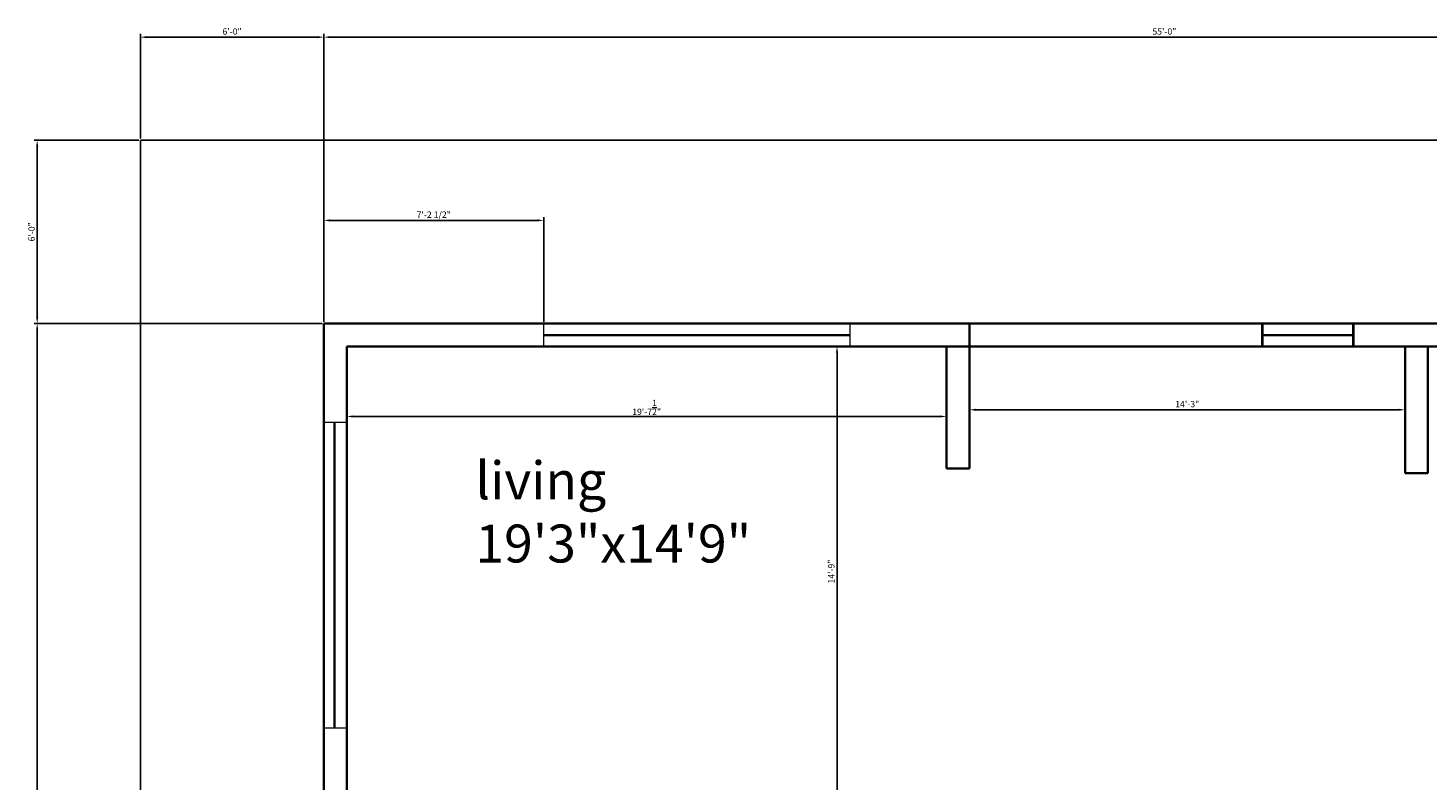
# Model space of a CAD drawing. Units: inches. Extents: x 250205121 to 250208111, y 89832590 to 89833271.
# Tile 7 of 14: x 250206174 to 250206724, y 89832964 to 89833259. Entities that reach past the tile are written whole.
import ezdxf

# ---------------------------------------------------------------- set-up
doc = ezdxf.new("R2010")
doc.units = ezdxf.units.IN
for name, color, linetype, lineweight in [('A-AREA-IDEN', 4, 'Continuous', 18), ('A-WALL', 7, 'Continuous', 35), ('C-PROP', 8, 'Continuous', 25), ('dimensions', 2, 'Continuous', 18), ('window', 4, 'Continuous', 18)]:
    doc.layers.add(name, color=color, linetype=linetype, lineweight=lineweight)
doc.styles.get("Standard").update_dxf_attribs({"font": 'arial.ttf'})
doc.dimstyles.new('ISO-25', dxfattribs={"dimtxt": 2.5, "dimasz": 2.5, "dimexe": 1.25, "dimexo": 0.625, "dimtad": 1, "dimlunit": 4, "dimtxsty": 'Standard', "dimcen": 2.5, "dimadec": 0, "dimazin": 0, "dimtfac": 1, "dimtmove": 0, "dimatfit": 3, "dimfxl": 1, "dimarcsym": 0})

# ---------------------------------------------------------------- blocks, each defined once
blk = doc.blocks.new('*D9')
at = {"layer": 'Defpoints', "color": 0, "transparency": 16777216}
for p in [(250206299.19, 89833113.08), (250206534.69, 89833113.08), (250206534.69, 89833106.78)]:
    blk.add_point(p, dxfattribs=at)
at = {"layer": 'dimensions', "color": 0, "lineweight": -2, "transparency": 16777216}
for p, q in [((250206299.19, 89833112.45), (250206299.19, 89833105.53)), ((250206534.69, 89833112.45), (250206534.69, 89833105.53)), ((250206301.69, 89833106.78), (250206532.19, 89833106.78))]:
    blk.add_line(p, q, dxfattribs=at)
at = {"layer": 'dimensions', "color": 0, "transparency": 16777216}
for points in [[(250206301.69, 89833107.19), (250206301.69, 89833106.36), (250206299.19, 89833106.78)], [(250206532.19, 89833107.19), (250206532.19, 89833106.36), (250206534.69, 89833106.78)]]:
    blk.add_solid(points, dxfattribs=at)
at = {"layer": 'dimensions', "color": 0, "transparency": 16777216, "insert": (250206416.94, 89833110.35), "char_height": 2.5, "attachment_point": 5}
blk.add_mtext('19\'-7{\\H1x;\\S1/2;}"', dxfattribs=at)
blk = doc.blocks.new('*D10')
at = {"layer": 'Defpoints', "color": 0, "transparency": 16777216}
for p in [(250206514.09, 89833134.33), (250206491.68, 89832957.33), (250206514.09, 89832957.33)]:
    blk.add_point(p, dxfattribs=at)
at = {"layer": 'dimensions', "color": 0, "lineweight": -2, "transparency": 16777216}
for p, q in [((250206513.46, 89833134.33), (250206490.43, 89833134.33)), ((250206491.68, 89833131.83), (250206491.68, 89832959.83)), ((250206513.46, 89832957.33), (250206490.43, 89832957.33))]:
    blk.add_line(p, q, dxfattribs=at)
at = {"layer": 'dimensions', "color": 0, "transparency": 16777216}
for points in [[(250206491.26, 89833131.83), (250206492.1, 89833131.83), (250206491.68, 89833134.33)], [(250206491.26, 89832959.83), (250206492.1, 89832959.83), (250206491.68, 89832957.33)]]:
    blk.add_solid(points, dxfattribs=at)
at = {"layer": 'dimensions', "color": 0, "transparency": 16777216, "insert": (250206489.78, 89833045.83), "char_height": 2.5, "attachment_point": 5, "rotation": 90}
blk.add_mtext('14\'-9"', dxfattribs=at)
blk = doc.blocks.new('*D11')
at = {"layer": 'Defpoints', "color": 0, "transparency": 16777216}
for p in [(250206543.69, 89833110.33), (250206714.69, 89833109.4), (250206714.69, 89833109.4)]:
    blk.add_point(p, dxfattribs=at)
at = {"layer": 'dimensions', "color": 0, "lineweight": -2, "transparency": 16777216}
for p, q in [((250206543.69, 89833109.7), (250206543.69, 89833108.15)), ((250206546.19, 89833109.4), (250206712.19, 89833109.4)), ((250206714.69, 89833110.03), (250206714.69, 89833110.65))]:
    blk.add_line(p, q, dxfattribs=at)
at = {"layer": 'dimensions', "color": 0, "transparency": 16777216}
for points in [[(250206546.19, 89833109.82), (250206546.19, 89833108.99), (250206543.69, 89833109.4)], [(250206712.19, 89833109.82), (250206712.19, 89833108.99), (250206714.69, 89833109.4)]]:
    blk.add_solid(points, dxfattribs=at)
at = {"layer": 'dimensions', "color": 0, "transparency": 16777216, "insert": (250206629.19, 89833111.31), "char_height": 2.5, "attachment_point": 5}
blk.add_mtext('14\'-3"', dxfattribs=at)
blk = doc.blocks.new('WIN-36IN')
for p, q in [((0, 0), (0, 36.08)), ((0, 36.08), (9, 36.08)), ((0, 35.58), (9, 35.58)), ((4.3, 35.58), (4.3, 0.5)), ((4.7, 35.58), (4.7, 0.5)), ((9, 36.08), (9, 0)), ((9, 0.5), (0, 0.5)), ((9, 0), (0, 0))]:
    blk.add_line(p, q)
blk = doc.blocks.new('WIN-120IN')
for p, q in [((0, 19), (0, 120.13)), ((0, 120.13), (9, 120.13)), ((4.1, 0), (4.1, 120.13)), ((4.5, 0), (4.5, 120.13)), ((9, 120.13), (9, 0)), ((0, 19), (0, 0)), ((9, 0), (0, 0))]:
    blk.add_line(p, q)
blk = doc.blocks.new('*D56')
at = {"layer": 'Defpoints', "color": 0, "transparency": 16777216}
for p in [(250206290.19, 89833255.83), (250206218.19, 89833215.33), (250206290.19, 89833143.33)]:
    blk.add_point(p, dxfattribs=at)
at = {"layer": 'dimensions', "color": 0, "lineweight": -2, "transparency": 16777216}
for p, q in [((250206218.19, 89833215.95), (250206218.19, 89833257.08)), ((250206220.69, 89833255.83), (250206287.69, 89833255.83)), ((250206290.19, 89833143.95), (250206290.19, 89833257.08))]:
    blk.add_line(p, q, dxfattribs=at)
at = {"layer": 'dimensions', "color": 0, "transparency": 16777216}
for points in [[(250206220.69, 89833256.24), (250206220.69, 89833255.41), (250206218.19, 89833255.83)], [(250206287.69, 89833256.24), (250206287.69, 89833255.41), (250206290.19, 89833255.83)]]:
    blk.add_solid(points, dxfattribs=at)
at = {"layer": 'dimensions', "color": 0, "transparency": 16777216, "insert": (250206254.19, 89833257.73), "char_height": 2.5, "attachment_point": 5}
blk.add_mtext('6\'-0"', dxfattribs=at)
blk = doc.blocks.new('*D57')
at = {"layer": 'Defpoints', "color": 0, "transparency": 16777216}
for p in [(250206177.69, 89833215.33), (250206218.19, 89833215.33), (250206290.19, 89833143.33)]:
    blk.add_point(p, dxfattribs=at)
at = {"layer": 'dimensions', "color": 0, "lineweight": -2, "transparency": 16777216}
for p, q in [((250206217.56, 89833215.33), (250206176.44, 89833215.33)), ((250206177.69, 89833145.83), (250206177.69, 89833212.83)), ((250206289.56, 89833143.33), (250206176.44, 89833143.33))]:
    blk.add_line(p, q, dxfattribs=at)
at = {"layer": 'dimensions', "color": 0, "transparency": 16777216}
for points in [[(250206177.27, 89833212.83), (250206178.1, 89833212.83), (250206177.69, 89833215.33)], [(250206177.27, 89833145.83), (250206178.1, 89833145.83), (250206177.69, 89833143.33)]]:
    blk.add_solid(points, dxfattribs=at)
at = {"layer": 'dimensions', "color": 0, "transparency": 16777216, "insert": (250206175.79, 89833179.33), "char_height": 2.5, "attachment_point": 5, "rotation": 90}
blk.add_mtext('6\'-0"', dxfattribs=at)
blk = doc.blocks.new('*D58')
at = {"layer": 'Defpoints', "color": 0, "transparency": 16777216}
for p in [(250206950.19, 89833255.83), (250206290.19, 89833143.33), (250206950.19, 89833143.33)]:
    blk.add_point(p, dxfattribs=at)
at = {"layer": 'dimensions', "color": 0, "lineweight": -2, "transparency": 16777216}
for p, q in [((250206290.19, 89833143.95), (250206290.19, 89833257.08)), ((250206292.69, 89833255.83), (250206947.69, 89833255.83)), ((250206950.19, 89833143.95), (250206950.19, 89833257.08))]:
    blk.add_line(p, q, dxfattribs=at)
at = {"layer": 'dimensions', "color": 0, "transparency": 16777216}
for points in [[(250206292.69, 89833256.24), (250206292.69, 89833255.41), (250206290.19, 89833255.83)], [(250206947.69, 89833256.24), (250206947.69, 89833255.41), (250206950.19, 89833255.83)]]:
    blk.add_solid(points, dxfattribs=at)
at = {"layer": 'dimensions', "color": 0, "transparency": 16777216, "insert": (250206620.19, 89833257.73), "char_height": 2.5, "attachment_point": 5}
blk.add_mtext('55\'-0"', dxfattribs=at)
blk = doc.blocks.new('*D59')
at = {"layer": 'Defpoints', "color": 0, "transparency": 16777216}
for p in [(250206177.69, 89833143.33), (250206290.19, 89833143.33), (250206290.19, 89832714.33)]:
    blk.add_point(p, dxfattribs=at)
at = {"layer": 'dimensions', "color": 0, "lineweight": -2, "transparency": 16777216}
for p, q in [((250206289.56, 89833143.33), (250206176.44, 89833143.33)), ((250206177.69, 89832716.83), (250206177.69, 89833140.83)), ((250206289.56, 89832714.33), (250206176.44, 89832714.33))]:
    blk.add_line(p, q, dxfattribs=at)
at = {"layer": 'dimensions', "color": 0, "transparency": 16777216}
for points in [[(250206177.27, 89833140.83), (250206178.1, 89833140.83), (250206177.69, 89833143.33)], [(250206177.27, 89832716.83), (250206178.1, 89832716.83), (250206177.69, 89832714.33)]]:
    blk.add_solid(points, dxfattribs=at)
at = {"layer": 'dimensions', "color": 0, "transparency": 16777216, "insert": (250206175.78, 89832928.83), "char_height": 2.5, "attachment_point": 5, "rotation": 90}
blk.add_mtext('35\'-9"', dxfattribs=at)
blk = doc.blocks.new('*D65')
at = {"layer": 'Defpoints', "color": 0, "transparency": 16777216}
for p in [(250206376.54, 89833183.83), (250206290.19, 89833143.33), (250206376.54, 89833143.33)]:
    blk.add_point(p, dxfattribs=at)
at = {"layer": 'dimensions', "color": 0, "lineweight": -2, "transparency": 16777216}
for p, q in [((250206290.19, 89833143.95), (250206290.19, 89833185.08)), ((250206292.69, 89833183.83), (250206374.04, 89833183.83)), ((250206376.54, 89833143.95), (250206376.54, 89833185.08))]:
    blk.add_line(p, q, dxfattribs=at)
at = {"layer": 'dimensions', "color": 0, "transparency": 16777216}
for points in [[(250206292.69, 89833184.24), (250206292.69, 89833183.41), (250206290.19, 89833183.83)], [(250206374.04, 89833184.24), (250206374.04, 89833183.41), (250206376.54, 89833183.83)]]:
    blk.add_solid(points, dxfattribs=at)
at = {"layer": 'dimensions', "color": 0, "transparency": 16777216, "insert": (250206333.36, 89833185.75), "char_height": 2.5, "attachment_point": 5}
blk.add_mtext('7\'-2 1/2"', dxfattribs=at)

msp = doc.modelspace()

# ---------------------------------------------------------------- linework, layer by layer
at = {"layer": 'A-WALL'}
for p, q in [((250206299.187, 89833143.328), (250206290.187, 89833143.328)), ((250206290.187, 89833143.328), (250206290.187, 89833134.328)), ((250206950.187, 89833143.328), (250206299.187, 89833143.328)), ((250206543.687, 89833134.328), (250206543.687, 89833143.328)), ((250206290.187, 89833134.328), (250206290.187, 89833091.828)), ((250206299.187, 89833134.328), (250206950.187, 89833134.328)), ((250206299.187, 89833134.328), (250206299.187, 89833091.828)), ((250206534.687, 89833086.328), (250206534.687, 89833134.328)), ((250206543.687, 89833134.328), (250206543.687, 89833086.328)), ((250206714.687, 89833084.481), (250206714.687, 89833134.328)), ((250206723.687, 89833084.481), (250206723.687, 89833134.328)), ((250206290.187, 89833091.828), (250206290.187, 89832714.328)), ((250206299.187, 89833091.828), (250206299.187, 89832723.328)), ((250206543.687, 89833086.328), (250206534.687, 89833086.328)), ((250206723.687, 89833084.481), (250206714.687, 89833084.481))]:
    msp.add_line(p, q, dxfattribs=at)
at = {"layer": 'C-PROP'}
for p, q in [((250206543.687, 89833215.328), (250206218.187, 89833215.328)), ((250206218.187, 89833215.328), (250206218.187, 89832642.328)), ((250207020.687, 89833215.328), (250206543.687, 89833215.328))]:
    msp.add_line(p, q, dxfattribs=at)

# ---------------------------------------------------------------- block references
at = {"layer": 'window'}
for name, p, rotation in [('WIN-120IN', (250206496.673, 89833134.328), 90.00000000304487), ('WIN-36IN', (250206694.527, 89833134.328), 89.99999987754511)]:
    msp.add_blockref(name, p, dxfattribs=dict(at, rotation=rotation))
msp.add_blockref('WIN-120IN', (250206290.187, 89832984.359), dxfattribs=at)

# ---------------------------------------------------------------- texts
at = {"layer": 'A-AREA-IDEN', "insert": (250206349.714, 89833089.097), "char_height": 14.88606, "attachment_point": 1}
msp.add_mtext_dynamic_manual_height_columns('living\\P19\'3"x14\'9"', width=23.63705, gutter_width=74.43, heights=[0], dxfattribs=at)

# ---------------------------------------------------------------- dimensions: what is measured, and where the dimension line sits
at = {"layer": 'dimensions'}
for base, p1, p2, override, picture, middle in [((250206290.187, 89833255.828), (250206218.187, 89833215.328), (250206290.187, 89833143.328), {"dimdec": 1, "dimlfac": 1, "dimrnd": 0, "dimzin": 1, "dimdsep": 46, "dimlunit": 4, "dimfrac": 2}, '*D56', (250206254.187, 89833257.729)), ((250206950.187, 89833255.828), (250206290.187, 89833143.328), (250206950.187, 89833143.328), {"dimdec": 1, "dimlfac": 1, "dimrnd": 0, "dimzin": 1, "dimdsep": 46, "dimlunit": 4, "dimfrac": 2}, '*D58', (250206620.187, 89833257.729)), ((250206534.687, 89833106.776), (250206299.187, 89833113.078), (250206534.687, 89833113.078), {"dimclrd": 0, "dimclre": 0, "dimclrt": 0}, '*D9', (250206416.937, 89833110.35)), ((250206714.687, 89833109.404), (250206543.687, 89833110.328), (250206714.687, 89833109.404), {"dimclrd": 0, "dimclre": 0, "dimclrt": 0}, '*D11', (250206629.187, 89833111.307))]:
    dim = msp.add_linear_dim(base=base, p1=p1, p2=p2, dimstyle='ISO-25', override=override, dxfattribs=at)
    dim.commit()
    dim.dimension.update_dxf_attribs({"geometry": picture, "text_midpoint": middle})
for base, p1, p2, angle, override, picture, middle in [((250206177.687, 89833215.328), (250206290.187, 89833143.328), (250206218.187, 89833215.328), 90, {"dimdec": 1, "dimlfac": 1, "dimrnd": 0, "dimzin": 1, "dimdsep": 46, "dimlunit": 4, "dimfrac": 2}, '*D57', (250206175.786, 89833179.328)), ((250206376.541, 89833183.828), (250206290.187, 89833143.328), (250206376.541, 89833143.328), 0, {"dimdec": 1, "dimlfac": 1, "dimrnd": 0, "dimzin": 1, "dimdsep": 46, "dimlunit": 4, "dimfrac": 2}, '*D65', (250206333.364, 89833185.746)), ((250206177.687, 89833143.328), (250206290.187, 89832714.328), (250206290.187, 89833143.328), 90, {"dimdec": 1, "dimlfac": 1, "dimrnd": 0, "dimzin": 1, "dimdsep": 46, "dimlunit": 4, "dimfrac": 2}, '*D59', (250206175.785, 89832928.828)), ((250206491.68, 89832957.328), (250206514.089, 89833134.328), (250206514.089, 89832957.328), 90, {"dimclrd": 0, "dimclre": 0, "dimclrt": 0}, '*D10', (250206489.778, 89833045.828))]:
    dim = msp.add_linear_dim(base=base, p1=p1, p2=p2, angle=angle, dimstyle='ISO-25', override=override, dxfattribs=at)
    dim.commit()
    dim.dimension.update_dxf_attribs({"geometry": picture, "text_midpoint": middle})

doc.saveas('drawing.dxf')
